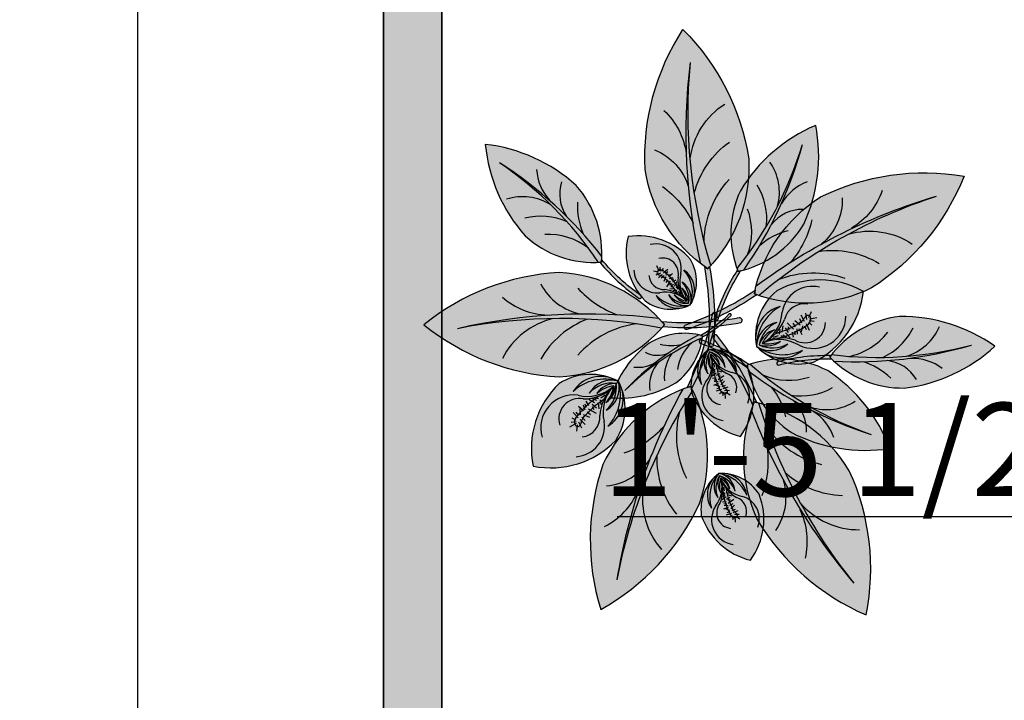
# Model space of a CAD drawing. Units: inches. Extents: x 3008 to 4088, y 1255 to 2137.
# Tile 6 of 30: x 3008 to 3093, y 1728 to 1787. Entities that reach past the tile are written whole.
import ezdxf

# ---------------------------------------------------------------- set-up
doc = ezdxf.new("R2010")
doc.units = ezdxf.units.IN
for name, color, linetype, lineweight in [('A-ANNO-DIMS', 2, 'Continuous', 18), ('C-PROP', 1, 'Continuous', 35), ('C-PROP-PATT', 9, 'Continuous', 13), ('L-PLNT', 3, 'Continuous', 13)]:
    doc.layers.add(name, color=color, linetype=linetype, lineweight=lineweight)
doc.layers.add('MESA', color=7, linetype='Continuous')
doc.styles.get("Standard").update_dxf_attribs({"font": 'arial.ttf'})
doc.dimstyles.new('ISO-25', dxfattribs={"dimtxt": 8, "dimasz": 2.5, "dimexe": 1.25, "dimexo": 0.625, "dimtad": 1, "dimdec": 1, "dimlunit": 3, "dimtxsty": 'Standard', "dimcen": 2.5, "dimadec": 0, "dimazin": 0, "dimtfac": 1, "dimtdec": 1, "dimtmove": 0, "dimatfit": 3, "dimfxl": 1, "dimarcsym": 0})

# ---------------------------------------------------------------- blocks, each defined once
blk = doc.blocks.new('*D2')
at = {"layer": 'A-ANNO-DIMS', "color": 0, "lineweight": -2, "transparency": 16777216}
for p, q in [((3039.040660450281, 2003.966263701819), (3017.259837783714, 2003.966263701819)), ((3018.509837783714, 2001.466263701819), (3018.509837783714, 1346.466263701818)), ((3039.040660450281, 1343.966263701819), (3017.259837783714, 1343.966263701819))]:
    blk.add_line(p, q, dxfattribs=at)
at = {"layer": 'A-ANNO-DIMS', "color": 0, "transparency": 16777216}
for points in [[(3018.093171117048, 2001.466263701819), (3018.926504450381, 2001.466263701819), (3018.509837783714, 2003.966263701819)], [(3018.093171117048, 1346.466263701818), (3018.926504450381, 1346.466263701818), (3018.509837783714, 1343.966263701819)]]:
    blk.add_solid(points, dxfattribs=at)
at = {"layer": 'Defpoints', "color": 0, "transparency": 16777216}
for p in [(3039.665660450281, 2003.966263701819), (3018.509837783714, 1343.966263701819), (3039.665660450281, 1343.966263701819)]:
    blk.add_point(p, dxfattribs=at)
at = {"layer": 'A-ANNO-DIMS', "color": 0, "transparency": 16777216, "insert": (3013.816624959703, 1673.966263701817), "char_height": 8, "attachment_point": 5, "rotation": 90}
blk.add_mtext("55'", dxfattribs=at)
blk = doc.blocks.new('folha Ant')
at = {"layer": 'MESA', "ltscale": 0.8}
h = blk.add_hatch(color=256, dxfattribs=at)
h.dxf.hatch_style = 1
h.set_gradient(color1=(103, 159, 96), color2=(179, 207, 175), one_color=1, tint=0.75, name='INVCURVED')
h.paths.add_polyline_path([(0.2265621468313839, 0.067551627434284, 0.1995123331975758), (0.098925864658554, 0.0067316513731726, 0.0967495278531692), (0.3533341132944088, 0.0074920887013263, -0.0866542067648319), (0.1023075862732412, -0.0052892013649171, 0.1924888780828613), (0.2265621468304744, -0.0624483725655409, 0.1586077411667837), (0.3952802919023952, 0.0025516274343431, 0.1586077411660197)])
h = blk.add_hatch(color=256, dxfattribs=at)
h.dxf.hatch_style = 1
h.set_gradient(color1=(179, 116, 77), color2=(114, 74, 49), one_color=1, tint=0.3199999928474426, name='CURVED')
h.paths.add_polyline_path([(0.0500009949356581, -0.0003325791788029), (0.0485055512837107, 0.0056977163088163, 0.0331076850617534), (0, -5.68e-14, 0.8090823413515374), (0.0019822352231813, -0.0060052531489987, -0.032777259300629)])
h.paths.add_polyline_path([(0.0973387667876296, 0.0049430375559041, 0.0331076850617478), (0.0485055512837107, 0.0056977163088163), (0.0500009949356581, -0.0003325791788029, -0.0327772593006016), (0.0983492748691788, -0.0009839943787711), (0.0952802919024407, 0.0025516274344568)])
h = blk.add_hatch(color=256, dxfattribs=at)
h.dxf.hatch_style = 1
h.set_gradient(color1=(103, 159, 96), color2=(52, 80, 48), one_color=1, tint=0.25)
h.paths.add_polyline_path([(0.353334113293613, 0.0074920887011558, -0.0967495278528606), (0.098925864658554, 0.0067316513732294, 0.0075274511230123), (0.095280291902327, 0.0025516274344, 0.01429188129495), (0.1023075862732412, -0.0052892013649171, 0.0866542067645507)])
blk.add_lwpolyline([(0.0983492748691788, -0.0009839943787711), (0.095280291902327, 0.0025516274344), (0.0973387667876296, 0.0049430375559041, 0.0662880296797218), (0, -5.68e-14, 0.8090823413515376), (0.0019822352231813, -0.0060052531489987, -0.0656250227609106)], format="xyb", close=True, dxfattribs=at)
for centre, radius, start, end in [((0.2359212193687199, -0.116427435949106), 0.1842169590516126, 92.91214396360807, 139.7695295797653), ((0.2110445794835414, -0.22419454821312), 0.2921585629436254, 50.90546460646405, 86.95538728132964), ((0.1143519570299531, 0.1191639001535236), 0.1187176334694229, 277.6411412097905, 318.4820087943453), ((0.1514763381197781, 0.1013313988557911), 0.1128992328564817, 290.5634166545446, 330.4539067144625), ((0.2122509936349388, 0.0879357745472476), 0.0955134836949057, 283.0012749323539, 333.1910720874903), ((0.2359212193687199, 0.1215306908179059), 0.1842169590516126, 220.2304704202346, 267.0878560363919), ((0.2241834180391606, 0.6583472640468245), 0.6635452971417175, 259.1189790274021, 281.2235391101338), ((0.1912233305980635, 0.7198824189188713), 0.7306024147604738, 263.0096624057024, 282.8198580038255), ((0.2110445794835414, 0.2292978030819199), 0.2921585629436254, 273.0446127186704, 309.0945353935359), ((0.1126560144376754, -0.1239479423437615), 0.1214242157519734, 41.75279468237299, 70.1060592868036), ((0.185327045767167, -0.0821234749886912), 0.072723812353325, 27.73755792858033, 79.23474605660121), ((0.2380907894142865, -0.0995343211653221), 0.0901952331959032, 48.80268108674044, 88.011030410351)]:
    blk.add_arc(centre, radius, start, end, dxfattribs=at)
blk = doc.blocks.new('folha A')
at = {"layer": 'MESA', "ltscale": 0.8}
h = blk.add_hatch(color=256, dxfattribs=at)
h.dxf.hatch_style = 1
h.set_gradient(color1=(237, 238, 238), one_color=1, tint=1)
h.paths.add_polyline_path([(0.1500000000024784, -7.6739e-12, 0.25690918051708), (0.0543124233674917, 0.0499999999922807, 0.2403030205165218), (0.0027820933477187, 0.0075036462510525, -0.3583807301859824), (0.0489413967899282, 0.03059436764255, 0.2702333190890776), (5.457e-12, -1.9327e-12, -0.3489770048102109), (0.0362881742687478, 0.014937604615227, 0.2509502793129825), (0.0039011655312606, -7.2191e-12, -0.2453890551403372), (0.0298115942678123, 0.0079955418688655, 0.1532458537889449), (0.0081856605954727, -6.8781e-12, 0.1518402250092038), (0.029600360026393, -0.0079843878059478, 0.0013736651199141), (0.0298115942676987, -0.0079955418812006, -0.245389055139057), (0.0039011655312606, -5.1728e-12, 0.2509502793127925), (0.0362881742687478, -0.014937604627562, -0.3489770048638718), (2.5011e-12, -5.1728e-12, 0.2702333191166405), (0.0489413967897008, -0.030594367654885, -0.358380731124288), (0.0027820932926943, -0.0075036461396394, 0.240303021013481), (0.054312423367378, -0.0500000000076852, 0.2569091805174252)])
edge = h.paths.add_edge_path(flags=16)
edge.add_arc((0.0097898024341703, 0.0552266440084282), 0.0552267033258632, 269.91602910653864, 271.41538979230364, ccw=False)
edge.add_arc((0.0109976306376893, -0.0487231262524688), 0.048740167733952, 89.8162517801581, 91.51516711851127, ccw=False)
edge.add_arc((0.0097898024345113, 0.055226644008485), 0.0552267033258632, 271.4153897919484, 288.9744624160262)
edge.add_spline(control_points=[(0.0278493569923057, 0.0029888582377566), (0.0280603768010224, 0.0029667323112221), (0.0300297853247003, 0.0027530242055605), (0.0319913285158009, 0.0024730861610465), (0.033739264015594, 0.0022193171533331)], knot_values=[0.2471511740125481, 0.2471511740125481, 0.2471511740125481, 0.2471511740125481, 0.247785628570655, 0.2530743171580143, 0.2530743171580143, 0.2530743171580143, 0.2530743171580143], degree=3, periodic=0)
edge.add_spline(control_points=[(0.033739264015594, 0.0022193171533331), (0.0349010022036964, 0.0020506535228719), (0.0360611952067984, 0.0018803040447324), (0.0372206570558547, 0.0017226504870109)], knot_values=[0.2436361292652643, 0.2436361292652643, 0.2436361292652643, 0.2436361292652643, 0.2471511740125481, 0.2471511740125481, 0.2471511740125481, 0.2471511740125481], degree=3, periodic=0)
edge.add_spline(control_points=[(0.0372206570558547, 0.0017226504870109), (0.0385458579326041, 0.00154246117512), (0.0404924684427215, 0.0013019665915976), (0.0424396413530985, 0.0011437083773558), (0.0430625787902272, 0.001100603847874)], knot_values=[0.2377304945037521, 0.2377304945037521, 0.2377304945037521, 0.2377304945037521, 0.2417479965750198, 0.2436361292652643, 0.2436361292652643, 0.2436361292652643, 0.2436361292652643], degree=3, periodic=0)
edge.add_spline(control_points=[(0.0430625787902272, 0.001100603847874), (0.0440233698390102, 0.0010341213351808), (0.0449850954752265, 0.0009854644238203), (0.0459489862383862, 0.000951284047062)], knot_values=[0.2348183224622999, 0.2348183224622999, 0.2348183224622999, 0.2348183224622999, 0.2377304945037521, 0.2377304945037521, 0.2377304945037521, 0.2377304945037521], degree=3, periodic=0)
edge.add_spline(control_points=[(0.0459489862383862, 0.000951284047062), (0.0472356690391962, 0.0009056571932433), (0.0485262099156216, 0.0008858263155958), (0.0498235358940065, 0.0008838251475822)], knot_values=[0.2309309092598198, 0.2309309092598198, 0.2309309092598198, 0.2309309092598198, 0.2348183224622999, 0.2348183224622999, 0.2348183224622999, 0.2348183224622999], degree=3, periodic=0)
edge.add_spline(control_points=[(0.0498235358940065, 0.0008838251475822), (0.051311952643232, 0.0008815292157465), (0.0528093005397068, 0.0009027023137946), (0.054319999895597, 0.0009353140121675)], knot_values=[0.2264708961110354, 0.2264708961110354, 0.2264708961110354, 0.2264708961110354, 0.2309309092598199, 0.2309309092598199, 0.2309309092598199, 0.2309309092598199], degree=3, periodic=0)
edge.add_spline(control_points=[(0.054319999895597, 0.0009353140121675), (0.0546767571066766, 0.0009430153847347), (0.0563551683278547, 0.0009821669427197), (0.058051274583363, 0.0010318868079935), (0.0593717098601019, 0.0011273838792363)], knot_values=[0.2215260703448321, 0.2215260703448321, 0.2215260703448321, 0.2215260703448321, 0.2225793188594869, 0.2264708961110354, 0.2264708961110354, 0.2264708961110354, 0.2264708961110354], degree=3, periodic=0)
edge.add_spline(control_points=[(0.0593717098601019, 0.0011273838792363), (0.0608505486812874, 0.0012343370778467), (0.0623113251667746, 0.0014119930674497), (0.0637184140251748, 0.0017303410663772)], knot_values=[0.2171676473178, 0.2171676473178, 0.2171676473178, 0.2171676473178, 0.2215260703448321, 0.2215260703448321, 0.2215260703448321, 0.2215260703448321], degree=3, periodic=0)
edge.add_spline(control_points=[(0.0637184140251748, 0.0017303410663772), (0.0647835272229713, 0.0019713184951229), (0.06603866541559, 0.002361556979622), (0.0672257540494457, 0.0029151988588296), (0.0674334326948838, 0.0030161580187382)], knot_values=[0.2131642620453263, 0.2131642620453263, 0.2131642620453263, 0.2131642620453263, 0.2164634238997696, 0.2171676473178, 0.2171676473178, 0.2171676473178, 0.2171676473178], degree=3, periodic=0)
edge.add_spline(control_points=[(0.0674334326948838, 0.0030161580187382), (0.0684934187318049, 0.0035314507664452), (0.0700375999888365, 0.0044431056608687), (0.0718040038906338, 0.0051196726092257), (0.0723976845548577, 0.0052385899649039)], knot_values=[0.2077773224475376, 0.2077773224475376, 0.2077773224475376, 0.2077773224475376, 0.2113716592103856, 0.2131642620453263, 0.2131642620453263, 0.2131642620453263, 0.2131642620453263], degree=3, periodic=0)
edge.add_spline(control_points=[(0.0723976845548577, 0.0052385899649039), (0.0729108187287011, 0.005341373435499), (0.0743578356647277, 0.0054068806913392), (0.0757446281196508, 0.0044472076547777), (0.076223593437021, 0.0036434068665585)], knot_values=[0.2034451630184741, 0.2034451630184741, 0.2034451630184741, 0.2034451630184741, 0.2049945578871382, 0.2077773224475375, 0.2077773224475375, 0.2077773224475375, 0.2077773224475375], degree=3, periodic=0)
edge.add_spline(control_points=[(0.076223593437021, 0.0036434068665585), (0.0762526630850289, 0.0035946221108247), (0.0768142944056081, 0.0025861272038696), (0.0767002674994046, 0.0011988541661481), (0.0763483320893101, 1.8759929219e-05), (0.0763162053667657, -8.15744999159e-05)], knot_values=[0.1996944706411438, 0.1996944706411438, 0.1996944706411438, 0.1996944706411438, 0.1998633638435843, 0.2031371852270858, 0.2034451630184741, 0.2034451630184741, 0.2034451630184741, 0.2034451630184741], degree=3, periodic=0)
edge.add_spline(control_points=[(0.0763162053667657, -8.15744999159e-05), (0.0760922549727639, -0.0007809902242002), (0.0756616910540515, -0.0016626883124218), (0.0750175512879423, -0.0023998413020081), (0.0748315435222367, -0.0025877827022214)], knot_values=[0.196756423636751, 0.196756423636751, 0.196756423636751, 0.196756423636751, 0.1989032889930779, 0.1996944706411438, 0.1996944706411438, 0.1996944706411438, 0.1996944706411438], degree=3, periodic=0)
edge.add_spline(control_points=[(0.0748315435222367, -0.0025877827022214), (0.0743082665363772, -0.0031164993883408), (0.0734373778385589, -0.0037391186011746), (0.0725002137970705, -0.0041944952659492), (0.0722284720523021, -0.0043124858620445)], knot_values=[0.1936429904609736, 0.1936429904609736, 0.1936429904609736, 0.1936429904609736, 0.1958687424163022, 0.1967564236367511, 0.1967564236367511, 0.1967564236367511, 0.1967564236367511], degree=3, periodic=0)
edge.add_spline(control_points=[(0.0722284720523021, -0.0043124858620445), (0.0708485967844581, -0.0049116293815814), (0.0693515594737164, -0.0052053922697155), (0.0678478270139067, -0.0054231344330447)], knot_values=[0.1891354409754396, 0.1891354409754396, 0.1891354409754396, 0.1891354409754396, 0.1936429904609736, 0.1936429904609736, 0.1936429904609736, 0.1936429904609736], degree=3, periodic=0)
edge.add_spline(control_points=[(0.0678478270139067, -0.0054231344330447), (0.06771109282829, -0.0054429336980206), (0.0666955122037507, -0.0055852647458892), (0.0656814581880099, -0.0057024537730399), (0.0648048099291145, -0.0057884767225573)], knot_values=[0.1860923947748148, 0.1860923947748148, 0.1860923947748148, 0.1860923947748148, 0.186502265629451, 0.1891354409754396, 0.1891354409754396, 0.1891354409754396, 0.1891354409754396], degree=3, periodic=0)
edge.add_spline(control_points=[(0.0648048099291145, -0.0057884767225573), (0.0634698784632519, -0.0059194696731311), (0.0621368526839206, -0.0060147950471787), (0.0608045983242391, -0.0060866121363574)], knot_values=[0.1820826809719926, 0.1820826809719926, 0.1820826809719926, 0.1820826809719926, 0.1860923947748149, 0.1860923947748149, 0.1860923947748149, 0.1860923947748149], degree=3, periodic=0)
edge.add_spline(control_points=[(0.0608045983242391, -0.0060866121363574), (0.0595780283853174, -0.0061527321546464), (0.0583521123309083, -0.0061989256613515), (0.0571259649824469, -0.0062346817291541)], knot_values=[0.1783910477803653, 0.1783910477803653, 0.1783910477803653, 0.1783910477803653, 0.1820826809719925, 0.1820826809719925, 0.1820826809719925, 0.1820826809719925], degree=3, periodic=0)
edge.add_spline(control_points=[(0.0571259649824469, -0.0062346817291541), (0.0567549493290471, -0.0062455010331064), (0.0555222126986337, -0.0062782721821009), (0.0542889716095942, -0.0063033964913188), (0.0534265626905608, -0.0063140481676669)], knot_values=[0.1746797876871894, 0.1746797876871894, 0.1746797876871894, 0.1746797876871894, 0.175796826109966, 0.1783910477803653, 0.1783910477803653, 0.1783910477803653, 0.1783910477803653], degree=3, periodic=0)
edge.add_spline(control_points=[(0.0534265626905608, -0.0063140481676669), (0.0524906151680398, -0.0063256081247687), (0.0515542477602367, -0.0063290287310451), (0.0506173198513125, -0.0063202526259261)], knot_values=[0.171864353741853, 0.171864353741853, 0.171864353741853, 0.171864353741853, 0.1746797876871893, 0.1746797876871893, 0.1746797876871893, 0.1746797876871893], degree=3, periodic=0)
edge.add_spline(control_points=[(0.0506173198513125, -0.0063202526259261), (0.0494177886716898, -0.0063090167436712), (0.048217338763493, -0.0062777889887116), (0.0470156750392334, -0.0062180548503648)], knot_values=[0.1682598066156458, 0.1682598066156458, 0.1682598066156458, 0.1682598066156458, 0.171864353741853, 0.171864353741853, 0.171864353741853, 0.171864353741853], degree=3, periodic=0)
edge.add_spline(control_points=[(0.0470156750392334, -0.0062180548503648), (0.0453335213580886, -0.0061344357823714), (0.0433578269695545, -0.0059708475257025), (0.041377747214824, -0.0056982907078122), (0.0410859622678572, -0.0056560847511946)], knot_values=[0.1623418216133555, 0.1623418216133555, 0.1623418216133555, 0.1623418216133555, 0.1673876610569998, 0.1682598066156458, 0.1682598066156458, 0.1682598066156458, 0.1682598066156458], degree=3, periodic=0)
edge.add_spline(control_points=[(0.0410859622678572, -0.0056560847511946), (0.0398520273901113, -0.0054775991836209), (0.0386185120281653, -0.0052626539931566), (0.0373943934592944, -0.0050360505769618)], knot_values=[0.1586535887747186, 0.1586535887747186, 0.1586535887747186, 0.1586535887747186, 0.1623418216133555, 0.1623418216133555, 0.1623418216133555, 0.1623418216133555], degree=3, periodic=0)
edge.add_spline(control_points=[(0.0373943934592944, -0.0050360505769618), (0.0365246595202962, -0.0048750492762792), (0.0356596691536879, -0.0047081628149499), (0.034802642192858, -0.0045442865819609)], knot_values=[0.1560331062850655, 0.1560331062850655, 0.1560331062850655, 0.1560331062850655, 0.1586535887747186, 0.1586535887747186, 0.1586535887747186, 0.1586535887747186], degree=3, periodic=0)
edge.add_spline(control_points=[(0.034802642192858, -0.0045442865819609), (0.0334719873470704, -0.0042898456909484), (0.0316821043800246, -0.00395248767353), (0.0299504285833336, -0.0036906648280137), (0.0294881583248525, -0.0036265151030079)], knot_values=[0.1504801710943955, 0.1504801710943955, 0.1504801710943955, 0.1504801710943955, 0.1545488385723417, 0.1560331062850655, 0.1560331062850655, 0.1560331062850655, 0.1560331062850655], degree=3, periodic=0)
edge.add_arc((0.0109976306373483, -0.0487231262524688), 0.0487401677339521, 67.70537335333205, 89.81625177975712)
h = blk.add_hatch(color=256, dxfattribs=at)
h.dxf.hatch_style = 1
h.set_gradient(color1=(117, 211, 105), one_color=1, tint=1)
h.paths.add_polyline_path([(0.0489413967899282, 0.03059436764255, 0.3583807301414101), (0.0027820933503335, 0.0075036462569074, 0.0272402125278007), (2.2737e-12, -8.0149e-12, -0.27023331912118)])
h.paths.add_polyline_path([(0.0039011655320564, -6.1391e-12, -0.2509502793036038), (0.0362881742687478, 0.014937604615227, 0.3489770048638718), (2.5011e-12, -7.1623e-12, 0.3489770048564635), (0.0362881742688615, -0.014937604627562, -0.2509502793046178)])
h.paths.add_polyline_path([(0.0298115942678123, 0.0079955418688655, 0.2453890551401661), (0.0039011655312606, -7.1623e-12, 0.2453890551330679), (0.0298115942676987, -0.0079955418812006, -0.1532458537798691), (0.0081856605964958, -6.1391e-12, -0.1532458537804744)], flags=17)
h.paths.add_polyline_path([(2.6148e-12, -5.1159e-12, 0.0272402124332956), (0.0027820933393059, -0.007503646244686, 0.3583807303279284), (0.0489413967898145, -0.030594367654885, -0.2702333191168038)])
h = blk.add_hatch(color=256, dxfattribs=at)
h.dxf.hatch_style = 1
h.set_gradient(color1=(68, 182, 53), color2=(121, 213, 109), one_color=1, tint=0.6299999952316285, name='CYLINDER')
edge = h.paths.add_edge_path()
edge.add_spline(control_points=[(0.0722284720523021, -0.0043124858620445), (0.0725002137970705, -0.0041944952659492), (0.0734373778385589, -0.0037391186011746), (0.0743082665363772, -0.0031164993883408), (0.0748315435222367, -0.0025877827022214)], knot_values=[0.1936429904609736, 0.1936429904609736, 0.1936429904609736, 0.1936429904609736, 0.1945306716814224, 0.1967564236367511, 0.1967564236367511, 0.1967564236367511, 0.1967564236367511], degree=3, periodic=0)
edge.add_spline(control_points=[(0.0748315435222367, -0.0025877827022214), (0.0750175512879423, -0.0023998413020081), (0.0756616910540515, -0.0016626883124218), (0.0760922549727639, -0.0007809902242002), (0.0763162053667657, -8.15744999159e-05)], knot_values=[0.1967564236367511, 0.1967564236367511, 0.1967564236367511, 0.1967564236367511, 0.197547605284817, 0.1996944706411439, 0.1996944706411439, 0.1996944706411439, 0.1996944706411439], degree=3, periodic=0)
edge.add_spline(control_points=[(0.0763162053667657, -8.15744999159e-05), (0.0763483320893101, 1.8759929219e-05), (0.0767002674994046, 0.0011988541661481), (0.0768142944056081, 0.0025861272038696), (0.0762526630850289, 0.0035946221108247), (0.076223593437021, 0.0036434068665585)], knot_values=[0.1996944706411439, 0.1996944706411439, 0.1996944706411439, 0.1996944706411439, 0.200002448432532, 0.2032762698160337, 0.2034451630184741, 0.2034451630184741, 0.2034451630184741, 0.2034451630184741], degree=3, periodic=0)
edge.add_spline(control_points=[(0.076223593437021, 0.0036434068665585), (0.0757446281196508, 0.0044472076547777), (0.0743578356647277, 0.0054068806913392), (0.0729108187287011, 0.005341373435499), (0.0723976845548577, 0.0052385899649039)], knot_values=[0.2034451630184741, 0.2034451630184741, 0.2034451630184741, 0.2034451630184741, 0.2062279275788734, 0.2077773224475376, 0.2077773224475376, 0.2077773224475376, 0.2077773224475376], degree=3, periodic=0)
edge.add_spline(control_points=[(0.0723976845548577, 0.0052385899649039), (0.0718040038906338, 0.0051196726092257), (0.0700375999888365, 0.0044431056608687), (0.0684934187318049, 0.0035314507664452), (0.0674334326948838, 0.0030161580187382)], knot_values=[0.2077773224475376, 0.2077773224475376, 0.2077773224475376, 0.2077773224475376, 0.2095699252824783, 0.2131642620453263, 0.2131642620453263, 0.2131642620453263, 0.2131642620453263], degree=3, periodic=0)
edge.add_spline(control_points=[(0.0674334326948838, 0.0030161580187382), (0.0672257540494457, 0.0029151988588296), (0.06603866541559, 0.002361556979622), (0.0647835272229713, 0.0019713184951229), (0.0637184140251748, 0.0017303410663772)], knot_values=[0.2131642620453263, 0.2131642620453263, 0.2131642620453263, 0.2131642620453263, 0.2138684854633567, 0.2171676473178, 0.2171676473178, 0.2171676473178, 0.2171676473178], degree=3, periodic=0)
edge.add_spline(control_points=[(0.0637184140251748, 0.0017303410663772), (0.0623113251667746, 0.0014119930674497), (0.0608505486812874, 0.0012343370778467), (0.0593717098601019, 0.0011273838792363)], knot_values=[0.2171676473178, 0.2171676473178, 0.2171676473178, 0.2171676473178, 0.2215260703448321, 0.2215260703448321, 0.2215260703448321, 0.2215260703448321], degree=3, periodic=0)
edge.add_spline(control_points=[(0.0593717098601019, 0.0011273838792363), (0.058051274583363, 0.0010318868079935), (0.0563551683278547, 0.0009821669427197), (0.0546767571066766, 0.0009430153847347), (0.054319999895597, 0.0009353140121675)], knot_values=[0.2215260703448321, 0.2215260703448321, 0.2215260703448321, 0.2215260703448321, 0.2254176475963805, 0.2264708961110354, 0.2264708961110354, 0.2264708961110354, 0.2264708961110354], degree=3, periodic=0)
edge.add_spline(control_points=[(0.054319999895597, 0.0009353140121675), (0.0528093005397068, 0.0009027023137946), (0.051311952643232, 0.0008815292157465), (0.0498235358940065, 0.0008838251475822)], knot_values=[0.2264708961110354, 0.2264708961110354, 0.2264708961110354, 0.2264708961110354, 0.2309309092598199, 0.2309309092598199, 0.2309309092598199, 0.2309309092598199], degree=3, periodic=0)
edge.add_spline(control_points=[(0.0498235358940065, 0.0008838251475822), (0.0485262099156216, 0.0008858263155958), (0.0472356690391962, 0.0009056571932433), (0.0459489862383862, 0.000951284047062)], knot_values=[0.2309309092598199, 0.2309309092598199, 0.2309309092598199, 0.2309309092598199, 0.2348183224622999, 0.2348183224622999, 0.2348183224622999, 0.2348183224622999], degree=3, periodic=0)
edge.add_spline(control_points=[(0.0459489862383862, 0.000951284047062), (0.0449850954752265, 0.0009854644238203), (0.0440233698390102, 0.0010341213351808), (0.0430625787902272, 0.001100603847874)], knot_values=[0.2348183224622999, 0.2348183224622999, 0.2348183224622999, 0.2348183224622999, 0.2377304945037521, 0.2377304945037521, 0.2377304945037521, 0.2377304945037521], degree=3, periodic=0)
edge.add_spline(control_points=[(0.0430625787902272, 0.001100603847874), (0.0424396413530985, 0.0011437083773558), (0.0404924684427215, 0.0013019665915976), (0.0385458579326041, 0.00154246117512), (0.0372206570558547, 0.0017226504870109)], knot_values=[0.2377304945037521, 0.2377304945037521, 0.2377304945037521, 0.2377304945037521, 0.2396186271939966, 0.2436361292652643, 0.2436361292652643, 0.2436361292652643, 0.2436361292652643], degree=3, periodic=0)
edge.add_spline(control_points=[(0.0372206570558547, 0.0017226504870109), (0.0360611952067984, 0.0018803040447324), (0.0349010022036964, 0.0020506535228719), (0.033739264015594, 0.0022193171533331)], knot_values=[0.2436361292652643, 0.2436361292652643, 0.2436361292652643, 0.2436361292652643, 0.2471511740125481, 0.2471511740125481, 0.2471511740125481, 0.2471511740125481], degree=3, periodic=0)
edge.add_spline(control_points=[(0.033739264015594, 0.0022193171533331), (0.0319913285158009, 0.0024730861610465), (0.0300297853247003, 0.0027530242055605), (0.0280603768010224, 0.0029667323112221), (0.0278493569923057, 0.0029888582377566)], knot_values=[0.2471511740125481, 0.2471511740125481, 0.2471511740125481, 0.2471511740125481, 0.2524398625999074, 0.2530743171580144, 0.2530743171580144, 0.2530743171580144, 0.2530743171580144], degree=3, periodic=0)
edge.add_arc((0.0109976306372346, 0.0487231262389401), 0.0487401677339521, 271.5151671116926, 290.2273514497534, ccw=False)
edge.add_arc((0.0109976306373483, -0.0487231262524688), 0.0487401677339521, 67.70537335303408, 88.48483288844102, ccw=False)
edge.add_spline(control_points=[(0.0294881583248525, -0.0036265151030079), (0.0299504285833336, -0.0036906648280137), (0.0316821043800246, -0.00395248767353), (0.0334719873470704, -0.0042898456909484), (0.034802642192858, -0.0045442865819609)], knot_values=[0.1504801710943955, 0.1504801710943955, 0.1504801710943955, 0.1504801710943955, 0.1519644388071193, 0.1560331062850655, 0.1560331062850655, 0.1560331062850655, 0.1560331062850655], degree=3, periodic=0)
edge.add_spline(control_points=[(0.034802642192858, -0.0045442865819609), (0.0356596691536879, -0.0047081628149499), (0.0365246595202962, -0.0048750492762792), (0.0373943934592944, -0.0050360505769618)], knot_values=[0.1560331062850655, 0.1560331062850655, 0.1560331062850655, 0.1560331062850655, 0.1586535887747186, 0.1586535887747186, 0.1586535887747186, 0.1586535887747186], degree=3, periodic=0)
edge.add_spline(control_points=[(0.0373943934592944, -0.0050360505769618), (0.0386185120281653, -0.0052626539931566), (0.0398520273901113, -0.0054775991836209), (0.0410859622678572, -0.0056560847511946)], knot_values=[0.1586535887747186, 0.1586535887747186, 0.1586535887747186, 0.1586535887747186, 0.1623418216133555, 0.1623418216133555, 0.1623418216133555, 0.1623418216133555], degree=3, periodic=0)
edge.add_spline(control_points=[(0.0410859622678572, -0.0056560847511946), (0.041377747214824, -0.0056982907078122), (0.0433578269695545, -0.0059708475257025), (0.0453335213580886, -0.0061344357823714), (0.0470156750392334, -0.0062180548503648)], knot_values=[0.1623418216133555, 0.1623418216133555, 0.1623418216133555, 0.1623418216133555, 0.1632139671720015, 0.1682598066156458, 0.1682598066156458, 0.1682598066156458, 0.1682598066156458], degree=3, periodic=0)
edge.add_spline(control_points=[(0.0470156750392334, -0.0062180548503648), (0.048217338763493, -0.0062777889887116), (0.0494177886716898, -0.0063090167436712), (0.0506173198513125, -0.0063202526259261)], knot_values=[0.1682598066156458, 0.1682598066156458, 0.1682598066156458, 0.1682598066156458, 0.171864353741853, 0.171864353741853, 0.171864353741853, 0.171864353741853], degree=3, periodic=0)
edge.add_spline(control_points=[(0.0506173198513125, -0.0063202526259261), (0.0515542477602367, -0.0063290287310451), (0.0524906151680398, -0.0063256081247687), (0.0534265626905608, -0.0063140481676669)], knot_values=[0.171864353741853, 0.171864353741853, 0.171864353741853, 0.171864353741853, 0.1746797876871894, 0.1746797876871894, 0.1746797876871894, 0.1746797876871894], degree=3, periodic=0)
edge.add_spline(control_points=[(0.0534265626905608, -0.0063140481676669), (0.0542889716095942, -0.0063033964913188), (0.0555222126986337, -0.0062782721821009), (0.0567549493290471, -0.0062455010331064), (0.0571259649824469, -0.0062346817291541)], knot_values=[0.1746797876871894, 0.1746797876871894, 0.1746797876871894, 0.1746797876871894, 0.1772740093575887, 0.1783910477803653, 0.1783910477803653, 0.1783910477803653, 0.1783910477803653], degree=3, periodic=0)
edge.add_spline(control_points=[(0.0571259649824469, -0.0062346817291541), (0.0583521123309083, -0.0061989256613515), (0.0595780283853174, -0.0061527321546464), (0.0608045983242391, -0.0060866121363574)], knot_values=[0.1783910477803653, 0.1783910477803653, 0.1783910477803653, 0.1783910477803653, 0.1820826809719925, 0.1820826809719925, 0.1820826809719925, 0.1820826809719925], degree=3, periodic=0)
edge.add_spline(control_points=[(0.0608045983242391, -0.0060866121363574), (0.0621368526839206, -0.0060147950471787), (0.0634698784632519, -0.0059194696731311), (0.0648048099291145, -0.0057884767225573)], knot_values=[0.1820826809719925, 0.1820826809719925, 0.1820826809719925, 0.1820826809719925, 0.1860923947748148, 0.1860923947748148, 0.1860923947748148, 0.1860923947748148], degree=3, periodic=0)
edge.add_spline(control_points=[(0.0648048099291145, -0.0057884767225573), (0.0656814581880099, -0.0057024537730399), (0.0666955122037507, -0.0055852647458892), (0.06771109282829, -0.0054429336980206), (0.0678478270139067, -0.0054231344330447)], knot_values=[0.1860923947748148, 0.1860923947748148, 0.1860923947748148, 0.1860923947748148, 0.1887255701208035, 0.1891354409754396, 0.1891354409754396, 0.1891354409754396, 0.1891354409754396], degree=3, periodic=0)
edge.add_spline(control_points=[(0.0678478270139067, -0.0054231344330447), (0.0693515594737164, -0.0052053922697155), (0.0708485967844581, -0.0049116293815814), (0.0722284720523021, -0.0043124858620445)], knot_values=[0.1891354409754396, 0.1891354409754396, 0.1891354409754396, 0.1891354409754396, 0.1936429904609736, 0.1936429904609736, 0.1936429904609736, 0.1936429904609736], degree=3, periodic=0)
for p, q in [((0.0299105082010556, -0.0007887538810678), (0.0235952339990036, 0.0002629394136875)), ((0.0323984218861142, 0.0003585478950185), (0.0358430615689258, 0.0051388866734783)), ((0.0367043736649748, 0.0010278072643928), (0.041392894102728, 0.0073378817443199)), ((0.0434681084230988, -0.002749196835623), (0.0427483193392391, 0.0040839524132821)), ((0.0455074093767962, -0.0006931453997367), (0.0465600058022346, 0.0032267170466866)), ((0.0506669123122947, -0.0021497888009776), (0.0476673853291914, 0.0086394705344333)), ((0.0545020337686992, -0.0005975369184057), (0.0538321581774426, 0.0050432781921472)), ((0.0603852823452371, -0.0013106346101495), (0.0571457749424553, 0.0064815845519206)), ((0.0636670944763864, -0.0002709670030754), (0.0638192697583691, 0.0056634113481095)), ((0.067433432705343, 0.0003402961420989), (0.067433432705343, 0.0088381928908348)), ((0.0709701384337223, 0.0010974880219692), (0.073580553220836, 0.0086699185521297)), ((0.0744226912312343, 0.0005085704808039), (0.083601295539097, -0.0023520932771248)), ((0.0744797569619777, 0.0023158351726806), (0.0808758362387607, 0.0071851299244372)), ((0.0330682974773708, -0.001744838694492), (0.0355560589871402, -0.0057603949107374)), ((0.035938779821322, -0.0021272726198163), (0.0384266935063806, -0.0070989136495427)), ((0.0399887727759278, -0.0017902122110058), (0.0422683584998822, -0.0098221775293155)), ((0.0474274049095129, -0.0046673366620098), (0.0458677604445939, -0.0105415012862977)), ((0.051248678415277, -0.0049955270600321), (0.0493349220690789, -0.0090109979877866)), ((0.0546262087988225, -0.0037082667488448), (0.0518666622353976, -0.0097023470954696)), ((0.0570855135308648, -0.00451748465332), (0.0572769500355435, -0.0126441202787078)), ((0.0629048484889836, -0.0035883510264512), (0.0578657162014906, -0.0095824313731328)), ((0.0648854097838694, -0.0043794877552159), (0.0645807548693256, -0.0097052469066625)), ((0.0679439807763629, -0.0029889429918057), (0.067584086234433, -0.0120998939456172)), ((0.0718122764442342, -0.0028569162931831), (0.0733279422527176, -0.0081576858951848)), ((0.0731091141972229, -0.0013361358911084), (0.0781347028845403, -0.0049881069548974))]:
    blk.add_line(p, q, dxfattribs=at)
for centre, radius, start, end in [((0.0702054725255721, -0.021762193614336), 0.0735010302158171, 102.4876359423993, 162.7776828012337), ((0.05671225017079, -0.0619684510075445), 0.11199416586583, 33.59497954719926, 91.2278360308839), ((0.0787582860352814, 0.001178711467162), 0.037790359601106, 48.94459180381986, 144.5333458640495), ((0.0507074537488279, -0.02667339942235), 0.0572949919432905, 91.76636101785736, 152.2544980832791), ((0.0399006027258793, -0.0090152479365315), 0.0406282857579686, 77.1426402064678, 158.3650061540138), ((0.0275418619235097, -0.0153613701258451), 0.0315361039128264, 73.89831961037032, 150.8495708938813), ((0.0340385609313216, -0.0227636835650742), 0.0377683450871499, 86.58524390803764, 142.9351488220486), ((0.0067361554278023, 0.0481714661850674), 0.0482631034134151, 273.5313007263508, 328.7109950801629), ((0.009789802434625, 0.0552266440085418), 0.0552267033259255, 269.9160291180983, 311.5613261238024), ((0.065484522559359, -0.0022658954200097), 0.0249917089679118, 51.9711829949073, 139.6849855414374), ((0.0245116561445684, -0.0208099897789111), 0.0292890422790084, 79.57472959496688, 134.7240405880906), ((0.0317359577491061, -0.0304535101567467), 0.0384971788119126, 92.865245661769, 127.7154849712638), ((0.0109976306373483, -0.0487231262524688), 0.0487401677339625, 43.37026979831881, 91.51516710447387), ((0.0507074537488279, 0.026673399410015), 0.0572949919432905, 207.7455019167209, 268.2336389821426), ((0.0275418619235097, 0.01536137011351), 0.0315361039128264, 209.1504291061187, 286.1016803896297), ((0.0702054725255721, 0.0217621935989882), 0.0735010302158171, 197.2223171987663, 257.5123640576006), ((0.0399006027258793, 0.0090152479241965), 0.0406282857579686, 201.6349938459861, 282.8573597935322), ((0.0340385609313216, 0.0227636835527392), 0.0377683450871499, 217.0648511779514, 273.4147560919624), ((0.0245116561445684, 0.0208099897665761), 0.0292890422790084, 225.2759594119094, 280.4252704050331), ((0.0317359577491061, 0.0304535101444117), 0.0384971788119126, 232.2845150287362, 267.134754338231), ((0.0067361554278023, -0.0481714661994488), 0.0482631034134235, 31.28900491989511, 86.46869927365576), ((0.05671225017079, 0.0619684509921967), 0.11199416586583, 268.7721639691161, 326.4050204528007), ((0.0676036048272408, -0.001142890729966), 0.0254455969684388, 213.6770178921663, 332.84146336245), ((0.0804246307012591, 0.0017314091068101), 0.0408601604971052, 217.4347997438042, 331.7322078727132)]:
    blk.add_arc(centre, radius, start, end, dxfattribs=at)
blk.add_open_spline([(0.0294881583248525, -0.0036265151030079), (0.0299504285833336, -0.0036906648280137), (0.0339214467404645, -0.004291067787733), (0.0429211279173387, -0.0063901960301109), (0.0551521839533962, -0.0063753416519035), (0.0655425247363155, -0.0059191266024641), (0.0723266295508438, -0.0046739009702037), (0.0754199937998692, -0.0022648361421034), (0.0766349994396478, 0.0004047905306948), (0.0768988947944536, 0.0036153916319677), (0.0738413800877424, 0.0058230755210502), (0.0702424644561006, 0.0046257095267492), (0.0648451640843177, 0.0012686733014675), (0.0543717506296844, 0.0008670820694761), (0.0416465532200618, 0.0007808754981511), (0.0325343106322862, 0.002481248516176), (0.0280603768010224, 0.0029667323112221), (0.0278493569923057, 0.0029888582377566)], degree=3, knots=[0.1504801710943955, 0.1504801710943955, 0.1504801710943955, 0.1504801710943955, 0.1519644388071193, 0.1632139671720015, 0.1772740093575887, 0.1887255701208035, 0.1945306716814224, 0.197547605284817, 0.200002448432532, 0.2032762698160337, 0.2062279275788734, 0.2095699252824783, 0.2138684854633567, 0.2254176475963805, 0.2396186271939966, 0.2524398625999074, 0.2530743171580144, 0.2530743171580144, 0.2530743171580144, 0.2530743171580144], dxfattribs=at)
blk = doc.blocks.new('Anturio Completa')
at = {"layer": 'MESA', "xscale": -1}
for p, rotation in [((0.038164816599874, -0.3934418212937203), 275.9103487005753), ((0.004688124415793, -0.3743032628411242), 209.3422747969654)]:
    blk.add_blockref('folha Ant', p, dxfattribs=dict(at, rotation=rotation))
at = {"layer": 'MESA'}
for name, p, xscale, yscale, zscale, rotation in [('folha Ant', (0.0395727317190904, -0.3603861081941773), 0.6875195991112988, 0.6875195991112988, 0.6875195991112988, 62.02852832027476), ('folha Ant', (-0.0544865625379316, -0.3355314546774935), 0.6875195991113106, 0.6875195991113106, 0.6875195991113106, 134.6123703789177), ('folha A', (0.0090774471967734, -0.3435514574847502), 0.7678141644548924, 0.7678141644548924, 0.7678141644548924, 132.2423739965673), ('folha Ant', (0.0599915804356215, -0.3565513211773919), 0.4588451896756128, 0.4588451896756128, 0.4588451896756128, 214.0760858842101), ('folha Ant', (0.0225462578581528, -0.3869492755299006), 0.6875195991113232, 0.6875195991113232, 0.6875195991113232, 329.7037252995857), ('folha Ant', (0.1178120217846299, -0.414439397344836), 0.6875195991112375, 0.6875195991112375, 0.6875195991112375, 3.732606609119443), ('folha A', (0.0322296485155675, -0.3991639714711255), 0.7678141644548587, 0.7678141644548587, 0.7678141644548587, 290.0444626994612), ('folha A', (0.0446221947787535, -0.5536580275510801), 0.7678141644548587, 0.7678141644548587, 0.7678141644548587, 290.0444626994612)]:
    blk.add_blockref(name, p, dxfattribs=dict(at, xscale=xscale, yscale=yscale, zscale=zscale, rotation=rotation))
for name, p, rotation in [('folha A', (0.0916540610597849, -0.3951196848045697), 27.20904127110871), ('folha Ant', (0.0721602323493471, -0.3655884559983065), 180), ('folha Ant', (0.0427962071474895, -0.355751804571355), 248.0349850699403), ('folha Ant', (0.0422774706713653, -0.3812807503523459), 297.7195320534174), ('folha A', (-0.0806384879487041, -0.4386582278959282), 224.8255080541778)]:
    blk.add_blockref(name, p, dxfattribs=dict(at, rotation=rotation))
blk = doc.blocks.new('*D72')
at = {"layer": 'A-ANNO-DIMS', "color": 0, "lineweight": -2, "transparency": 16777216}
for p, q in [((3102.66566045028, 1735.292622111312), (3102.66566045028, 1745.366446111313)), ((3120.38220545028, 1735.292622111312), (3120.38220545028, 1745.366446111313)), ((3102.66566045028, 1744.116446111312), (3059.761499468015, 1744.116446111312)), ((3117.88220545028, 1744.116446111312), (3105.16566045028, 1744.116446111312))]:
    blk.add_line(p, q, dxfattribs=at)
at = {"layer": 'A-ANNO-DIMS', "color": 0, "transparency": 16777216}
for points in [[(3105.16566045028, 1744.533112777979), (3105.16566045028, 1743.699779444646), (3102.66566045028, 1744.116446111312)], [(3117.88220545028, 1744.533112777979), (3117.88220545028, 1743.699779444646), (3120.38220545028, 1744.116446111312)]]:
    blk.add_solid(points, dxfattribs=at)
at = {"layer": 'Defpoints', "color": 0, "transparency": 16777216}
for p in [(3102.66566045028, 1744.116446111312), (3102.66566045028, 1734.667622111312), (3120.38220545028, 1734.667622111312)]:
    blk.add_point(p, dxfattribs=at)
at = {"layer": 'A-ANNO-DIMS', "color": 0, "transparency": 16777216, "insert": (3079.963579959148, 1748.877871759334), "char_height": 8, "attachment_point": 5}
blk.add_mtext('1\'-5 1/2"', dxfattribs=at)

msp = doc.modelspace()

# ---------------------------------------------------------------- hatches: boundary and pattern name
at = {"layer": 'C-PROP-PATT'}
h = msp.add_hatch(color=256, dxfattribs=at)
h.dxf.hatch_style = 1
h.paths.add_polyline_path([(3519.66566045028, 2003.966263701818), (3039.66566045028, 2003.966263701818), (3039.66566045028, 1343.966263701818), (3051.66566045028, 1343.966263701818), (3051.66566045028, 1348.966263701818), (3044.66566045028, 1348.966263701818), (3044.66566045028, 1998.966263701818), (3514.66566045028, 1998.966263701818), (3514.66566045028, 1348.966263701818), (3219.665660450281, 1348.966263701818), (3219.66566045028, 1343.966263701818), (3519.66566045028, 1343.966263701818)])

# ---------------------------------------------------------------- linework, layer by layer
at = {"layer": 'C-PROP'}
for p, q in [((3039.66566045028, 1343.966263701818), (3039.66566045028, 2003.966263701818)), ((3044.66566045028, 1348.966263701818), (3044.66566045028, 1998.966263701818))]:
    msp.add_line(p, q, dxfattribs=at)

# ---------------------------------------------------------------- block references
at = {"layer": 'L-PLNT', "xscale": 68.94981777915199, "yscale": 68.94981777915199, "zscale": 68.94981777915199}
msp.add_blockref('Anturio Completa', (3065.411836173471, 1786.02607345099), dxfattribs=at)

# ---------------------------------------------------------------- dimensions: what is measured, and where the dimension line sits
at = {"layer": 'A-ANNO-DIMS'}
for base, p1, p2, angle, override, picture, middle in [((3018.509837783714, 1343.966263701819), (3039.66566045028, 2003.966263701818), (3039.66566045028, 1343.966263701818), 90, {"dimclrd": 0, "dimclre": 0, "dimclrt": 0}, '*D2', (3013.816624959703, 1673.966263701817)), ((3102.66566045028, 1744.116446111312), (3120.38220545028, 1734.667622111312), (3102.66566045028, 1734.667622111312), 180, {"dimdec": 1, "dimrnd": 0, "dimzin": 1, "dimlunit": 4, "dimfrac": 2}, '*D72', (3079.963579959148, 1748.877871759334))]:
    dim = msp.add_linear_dim(base=base, p1=p1, p2=p2, angle=angle, dimstyle='ISO-25', override=override, dxfattribs=at)
    dim.commit()
    dim.dimension.update_dxf_attribs({"geometry": picture, "text_midpoint": middle})

doc.saveas('drawing.dxf')
